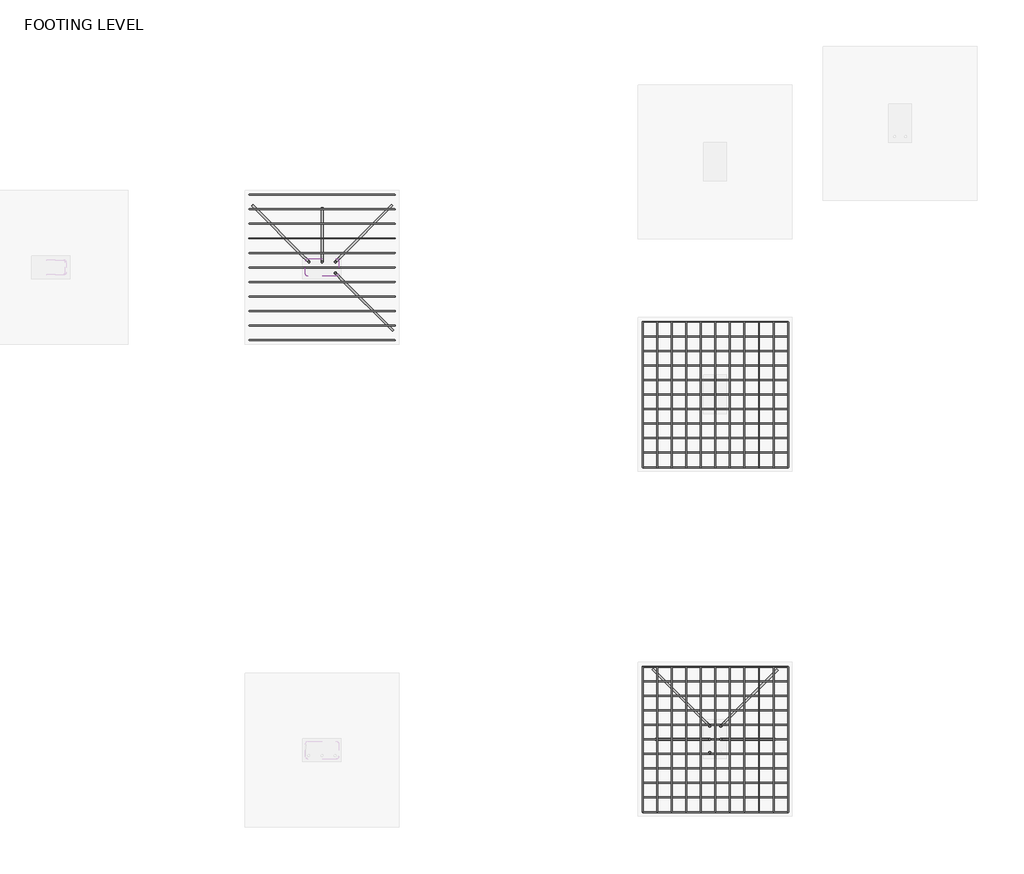
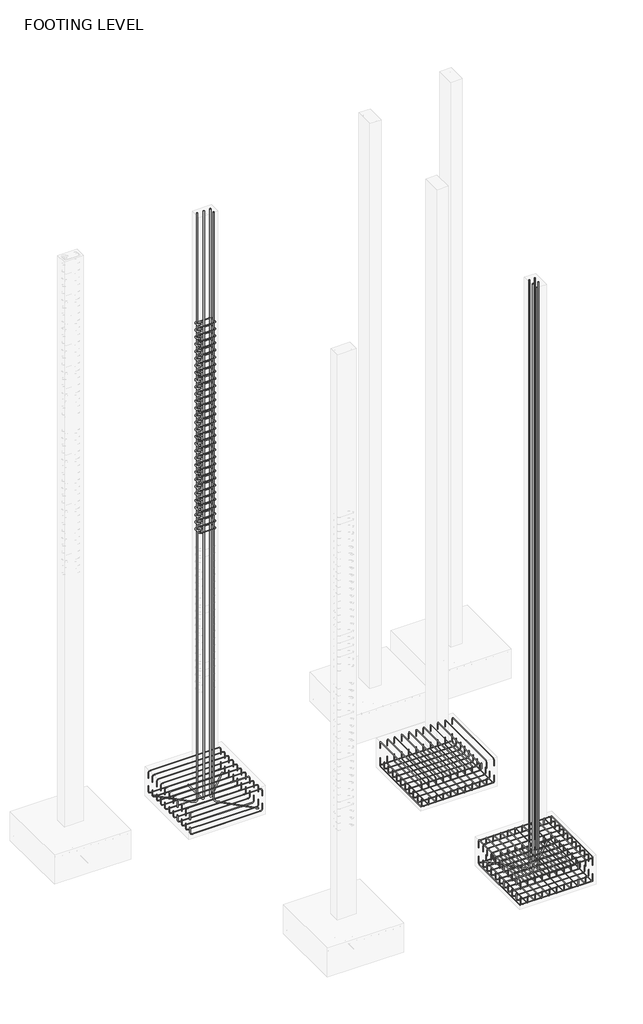
# One storey, part 5 of 10: 21 reinforcing bars.
"""IFC4 building model written with IfcOpenShell, lengths in millimetres."""

from ifc_helpers import new_model, si_unit, point, frame, origin, place, context, project, spatial, polyline, circle_curve, trimmed, segment, composite_curve, source, transform, mapped, element, save
from ifc_brep_helpers import swept_disk

model = new_model("IFC4")

# Units and contexts
model_context = context("Model", 3, world=origin())
ifc_project = project(units=[si_unit("LENGTHUNIT", "METRE", prefix="MILLI")], contexts=[model_context])

# Site, building, storey
site = spatial("IfcSite", under=ifc_project)
building = spatial("IfcBuilding", under=site)
storey = spatial("IfcBuildingStorey", under=building, Name="FOOTING LEVEL", Elevation=-1371.6)

# Reinforcing bars
placement = place(None, origin())
reinforcing_bar_shape = source(origin(), model_context, "Body", "SolidModel", [
    swept_disk(composite_curve([segment(polyline([(-7030.6793223, 2952.1203802, -1562.1), (-7030.6793223, 2952.1203802, -1447.8)]), True, "CONTINUOUS"), segment(trimmed(circle_curve(frame((-7030.6793223, 2985.4578802, -1447.8), z_axis=(-1.0, 0.0, 0.0), x_axis=(0.0, -33.33750000000009, 0.0)), 33.3375), [point((-7030.6793223, 2952.1203802, -1447.8))], [point((-7030.6793223, 2985.4578802, -1414.4625))], True, "CARTESIAN"), True, "CONTINUOUS"), segment(polyline([(-7030.6793223, 2985.4578802, -1414.4625), (-7030.6793223, 4357.0578802, -1414.4625)]), True, "CONTINUOUS"), segment(trimmed(circle_curve(frame((-7030.6793223, 4357.0578802, -1447.8), z_axis=(-1.0, 0.0, 0.0), x_axis=(0.0, 0.0, 33.337499999999864)), 33.3375), [point((-7030.6793223, 4357.0578802, -1414.4625))], [point((-7030.6793223, 4390.3953802, -1447.8))], True, "CARTESIAN"), True, "CONTINUOUS"), segment(polyline([(-7030.6793223, 4390.3953802, -1447.8), (-7030.6793223, 4390.3953802, -1562.1)]), True, "CONTINUOUS")], self_intersect=False), 4.7625),
])
element("IfcReinforcingBar", 1, at=placement, inside=storey, context=model_context, shape_type="MappedRepresentation", body=[
    mapped(reinforcing_bar_shape, transform((0.0, 0.0, 0.0), x_axis=(1.0, 0.0, 0.0), y_axis=(0.0, 1.0, 0.0), z_axis=(0.0, 0.0, 1.0))),
    mapped(reinforcing_bar_shape, transform((143.8275, 0.0, 0.0), x_axis=(1.0, 0.0, 0.0), y_axis=(0.0, 1.0, 0.0), z_axis=(0.0, 0.0, 1.0))),
    mapped(reinforcing_bar_shape, transform((287.655, 0.0, 0.0), x_axis=(1.0, 0.0, 0.0), y_axis=(0.0, 1.0, 0.0), z_axis=(0.0, 0.0, 1.0))),
    mapped(reinforcing_bar_shape, transform((431.4825, 0.0, 0.0), x_axis=(1.0, 0.0, 0.0), y_axis=(0.0, 1.0, 0.0), z_axis=(0.0, 0.0, 1.0))),
    mapped(reinforcing_bar_shape, transform((575.31, 0.0, 0.0), x_axis=(1.0, 0.0, 0.0), y_axis=(0.0, 1.0, 0.0), z_axis=(0.0, 0.0, 1.0))),
    mapped(reinforcing_bar_shape, transform((719.1375, 0.0, 0.0), x_axis=(1.0, 0.0, 0.0), y_axis=(0.0, 1.0, 0.0), z_axis=(0.0, 0.0, 1.0))),
    mapped(reinforcing_bar_shape, transform((862.965, 0.0, 0.0), x_axis=(1.0, 0.0, 0.0), y_axis=(0.0, 1.0, 0.0), z_axis=(0.0, 0.0, 1.0))),
    mapped(reinforcing_bar_shape, transform((1006.7925, 0.0, 0.0), x_axis=(1.0, 0.0, 0.0), y_axis=(0.0, 1.0, 0.0), z_axis=(0.0, 0.0, 1.0))),
    mapped(reinforcing_bar_shape, transform((1150.62, 0.0, 0.0), x_axis=(1.0, 0.0, 0.0), y_axis=(0.0, 1.0, 0.0), z_axis=(0.0, 0.0, 1.0))),
    mapped(reinforcing_bar_shape, transform((1294.4475, 0.0, 0.0), x_axis=(1.0, 0.0, 0.0), y_axis=(0.0, 1.0, 0.0), z_axis=(0.0, 0.0, 1.0))),
    mapped(reinforcing_bar_shape, transform((1438.275, 0.0, 0.0), x_axis=(1.0, 0.0, 0.0), y_axis=(0.0, 1.0, 0.0), z_axis=(0.0, 0.0, 1.0))),
])
reinforcing_bar_2_shape = source(origin(), model_context, "Body", "SolidModel", [
    swept_disk(composite_curve([segment(polyline([(-7030.6793223, 4390.3953802, -1790.7), (-7030.6793223, 4390.3953802, -1905.0)]), True, "CONTINUOUS"), segment(trimmed(circle_curve(frame((-7030.6793223, 4357.0578802, -1905.0), z_axis=(-1.0, 0.0, 0.0), x_axis=(0.0, 33.337499999999636, 0.0)), 33.3375), [point((-7030.6793223, 4390.3953802, -1905.0))], [point((-7030.6793223, 4357.0578802, -1938.3375))], True, "CARTESIAN"), True, "CONTINUOUS"), segment(polyline([(-7030.6793223, 4357.0578802, -1938.3375), (-7030.6793223, 2985.4578802, -1938.3375)]), True, "CONTINUOUS"), segment(trimmed(circle_curve(frame((-7030.6793223, 2985.4578802, -1905.0), z_axis=(-1.0, 0.0, 0.0), x_axis=(0.0, 0.0, -33.33750000000009)), 33.3375), [point((-7030.6793223, 2985.4578802, -1938.3375))], [point((-7030.6793223, 2952.1203802, -1905.0))], True, "CARTESIAN"), True, "CONTINUOUS"), segment(polyline([(-7030.6793223, 2952.1203802, -1905.0), (-7030.6793223, 2952.1203802, -1790.7)]), True, "CONTINUOUS")], self_intersect=False), 4.7625),
])
element("IfcReinforcingBar", 2, at=placement, inside=storey, context=model_context, shape_type="MappedRepresentation", body=[
    mapped(reinforcing_bar_2_shape, transform((0.0, 0.0, 0.0), x_axis=(1.0, 0.0, 0.0), y_axis=(0.0, 1.0, 0.0), z_axis=(0.0, 0.0, 1.0))),
    mapped(reinforcing_bar_2_shape, transform((143.8275, 0.0, 0.0), x_axis=(1.0, 0.0, 0.0), y_axis=(0.0, 1.0, 0.0), z_axis=(0.0, 0.0, 1.0))),
    mapped(reinforcing_bar_2_shape, transform((287.655, 0.0, 0.0), x_axis=(1.0, 0.0, 0.0), y_axis=(0.0, 1.0, 0.0), z_axis=(0.0, 0.0, 1.0))),
    mapped(reinforcing_bar_2_shape, transform((431.4825, 0.0, 0.0), x_axis=(1.0, 0.0, 0.0), y_axis=(0.0, 1.0, 0.0), z_axis=(0.0, 0.0, 1.0))),
    mapped(reinforcing_bar_2_shape, transform((575.31, 0.0, 0.0), x_axis=(1.0, 0.0, 0.0), y_axis=(0.0, 1.0, 0.0), z_axis=(0.0, 0.0, 1.0))),
    mapped(reinforcing_bar_2_shape, transform((719.1375, 0.0, 0.0), x_axis=(1.0, 0.0, 0.0), y_axis=(0.0, 1.0, 0.0), z_axis=(0.0, 0.0, 1.0))),
    mapped(reinforcing_bar_2_shape, transform((862.965, 0.0, 0.0), x_axis=(1.0, 0.0, 0.0), y_axis=(0.0, 1.0, 0.0), z_axis=(0.0, 0.0, 1.0))),
    mapped(reinforcing_bar_2_shape, transform((1006.7925, 0.0, 0.0), x_axis=(1.0, 0.0, 0.0), y_axis=(0.0, 1.0, 0.0), z_axis=(0.0, 0.0, 1.0))),
    mapped(reinforcing_bar_2_shape, transform((1150.62, 0.0, 0.0), x_axis=(1.0, 0.0, 0.0), y_axis=(0.0, 1.0, 0.0), z_axis=(0.0, 0.0, 1.0))),
    mapped(reinforcing_bar_2_shape, transform((1294.4475, 0.0, 0.0), x_axis=(1.0, 0.0, 0.0), y_axis=(0.0, 1.0, 0.0), z_axis=(0.0, 0.0, 1.0))),
    mapped(reinforcing_bar_2_shape, transform((1438.275, 0.0, 0.0), x_axis=(1.0, 0.0, 0.0), y_axis=(0.0, 1.0, 0.0), z_axis=(0.0, 0.0, 1.0))),
])
reinforcing_bar_3_shape = source(origin(), model_context, "Body", "SolidModel", [
    swept_disk(composite_curve([segment(polyline([(-5592.4043223, 4390.3953802, -1770.864029), (-5592.4043223, 4390.3953802, -1885.164029)]), True, "CONTINUOUS"), segment(trimmed(circle_curve(frame((-5625.7418223, 4390.3953802, -1885.164029), z_axis=(0.0, 1.0, 0.0), x_axis=(33.337500000000546, 0.0, 0.0)), 33.3375), [point((-5592.4043223, 4390.3953802, -1885.164029))], [point((-5625.7418223, 4390.3953802, -1918.501529))], True, "CARTESIAN"), True, "CONTINUOUS"), segment(polyline([(-5625.7418223, 4390.3953802, -1918.501529), (-6997.3418223, 4390.3953802, -1918.501529)]), True, "CONTINUOUS"), segment(trimmed(circle_curve(frame((-6997.3418223, 4390.3953802, -1885.164029), z_axis=(0.0, 1.0, 0.0), x_axis=(0.0, 0.0, -33.337499999999864)), 33.3375), [point((-6997.3418223, 4390.3953802, -1918.501529))], [point((-7030.6793223, 4390.3953802, -1885.164029))], True, "CARTESIAN"), True, "CONTINUOUS"), segment(polyline([(-7030.6793223, 4390.3953802, -1885.164029), (-7030.6793223, 4390.3953802, -1770.864029)]), True, "CONTINUOUS")], self_intersect=False), 4.7625),
])
element("IfcReinforcingBar", 3, at=placement, inside=storey, context=model_context, shape_type="MappedRepresentation", body=[
    mapped(reinforcing_bar_3_shape, transform((0.0, 0.0, 0.0), x_axis=(1.0, 0.0, 0.0), y_axis=(0.0, 1.0, 0.0), z_axis=(0.0, 0.0, 1.0))),
    mapped(reinforcing_bar_3_shape, transform((0.0, -143.8275, 0.0), x_axis=(1.0, 0.0, 0.0), y_axis=(0.0, 1.0, 0.0), z_axis=(0.0, 0.0, 1.0))),
    mapped(reinforcing_bar_3_shape, transform((0.0, -287.655, 0.0), x_axis=(1.0, 0.0, 0.0), y_axis=(0.0, 1.0, 0.0), z_axis=(0.0, 0.0, 1.0))),
    mapped(reinforcing_bar_3_shape, transform((0.0, -431.4825, 0.0), x_axis=(1.0, 0.0, 0.0), y_axis=(0.0, 1.0, 0.0), z_axis=(0.0, 0.0, 1.0))),
    mapped(reinforcing_bar_3_shape, transform((0.0, -575.31, 0.0), x_axis=(1.0, 0.0, 0.0), y_axis=(0.0, 1.0, 0.0), z_axis=(0.0, 0.0, 1.0))),
    mapped(reinforcing_bar_3_shape, transform((0.0, -719.1375, 0.0), x_axis=(1.0, 0.0, 0.0), y_axis=(0.0, 1.0, 0.0), z_axis=(0.0, 0.0, 1.0))),
    mapped(reinforcing_bar_3_shape, transform((0.0, -862.965, 0.0), x_axis=(1.0, 0.0, 0.0), y_axis=(0.0, 1.0, 0.0), z_axis=(0.0, 0.0, 1.0))),
    mapped(reinforcing_bar_3_shape, transform((0.0, -1006.7925, 0.0), x_axis=(1.0, 0.0, 0.0), y_axis=(0.0, 1.0, 0.0), z_axis=(0.0, 0.0, 1.0))),
    mapped(reinforcing_bar_3_shape, transform((0.0, -1150.62, 0.0), x_axis=(1.0, 0.0, 0.0), y_axis=(0.0, 1.0, 0.0), z_axis=(0.0, 0.0, 1.0))),
    mapped(reinforcing_bar_3_shape, transform((0.0, -1294.4475, 0.0), x_axis=(1.0, 0.0, 0.0), y_axis=(0.0, 1.0, 0.0), z_axis=(0.0, 0.0, 1.0))),
    mapped(reinforcing_bar_3_shape, transform((0.0, -1438.275, 0.0), x_axis=(1.0, 0.0, 0.0), y_axis=(0.0, 1.0, 0.0), z_axis=(0.0, 0.0, 1.0))),
])
reinforcing_bar_4_shape = source(origin(), model_context, "Body", "SolidModel", [
    swept_disk(composite_curve([segment(polyline([(-7030.6793223, -457.8296198, -1562.1), (-7030.6793223, -457.8296198, -1447.8)]), True, "CONTINUOUS"), segment(trimmed(circle_curve(frame((-7030.6793223, -424.4921198, -1447.8), z_axis=(-1.0, 0.0, 0.0), x_axis=(0.0, -33.33749999999998, 0.0)), 33.3375), [point((-7030.6793223, -457.8296198, -1447.8))], [point((-7030.6793223, -424.4921198, -1414.4625))], True, "CARTESIAN"), True, "CONTINUOUS"), segment(polyline([(-7030.6793223, -424.4921198, -1414.4625), (-7030.6793223, 947.1078802, -1414.4625)]), True, "CONTINUOUS"), segment(trimmed(circle_curve(frame((-7030.6793223, 947.1078802, -1447.8), z_axis=(-1.0, 0.0, 0.0), x_axis=(0.0, 0.0, 33.337499999999864)), 33.3375), [point((-7030.6793223, 947.1078802, -1414.4625))], [point((-7030.6793223, 980.4453802, -1447.8))], True, "CARTESIAN"), True, "CONTINUOUS"), segment(polyline([(-7030.6793223, 980.4453802, -1447.8), (-7030.6793223, 980.4453802, -1562.1)]), True, "CONTINUOUS")], self_intersect=False), 4.7625),
])
element("IfcReinforcingBar", 4, at=placement, inside=storey, context=model_context, shape_type="MappedRepresentation", body=[
    mapped(reinforcing_bar_4_shape, transform((0.0, 0.0, 0.0), x_axis=(1.0, 0.0, 0.0), y_axis=(0.0, 1.0, 0.0), z_axis=(0.0, 0.0, 1.0))),
    mapped(reinforcing_bar_4_shape, transform((143.8275, 0.0, 0.0), x_axis=(1.0, 0.0, 0.0), y_axis=(0.0, 1.0, 0.0), z_axis=(0.0, 0.0, 1.0))),
    mapped(reinforcing_bar_4_shape, transform((287.655, 0.0, 0.0), x_axis=(1.0, 0.0, 0.0), y_axis=(0.0, 1.0, 0.0), z_axis=(0.0, 0.0, 1.0))),
    mapped(reinforcing_bar_4_shape, transform((431.4825, 0.0, 0.0), x_axis=(1.0, 0.0, 0.0), y_axis=(0.0, 1.0, 0.0), z_axis=(0.0, 0.0, 1.0))),
    mapped(reinforcing_bar_4_shape, transform((575.31, 0.0, 0.0), x_axis=(1.0, 0.0, 0.0), y_axis=(0.0, 1.0, 0.0), z_axis=(0.0, 0.0, 1.0))),
    mapped(reinforcing_bar_4_shape, transform((719.1375, 0.0, 0.0), x_axis=(1.0, 0.0, 0.0), y_axis=(0.0, 1.0, 0.0), z_axis=(0.0, 0.0, 1.0))),
    mapped(reinforcing_bar_4_shape, transform((862.965, 0.0, 0.0), x_axis=(1.0, 0.0, 0.0), y_axis=(0.0, 1.0, 0.0), z_axis=(0.0, 0.0, 1.0))),
    mapped(reinforcing_bar_4_shape, transform((1006.7925, 0.0, 0.0), x_axis=(1.0, 0.0, 0.0), y_axis=(0.0, 1.0, 0.0), z_axis=(0.0, 0.0, 1.0))),
    mapped(reinforcing_bar_4_shape, transform((1150.62, 0.0, 0.0), x_axis=(1.0, 0.0, 0.0), y_axis=(0.0, 1.0, 0.0), z_axis=(0.0, 0.0, 1.0))),
    mapped(reinforcing_bar_4_shape, transform((1294.4475, 0.0, 0.0), x_axis=(1.0, 0.0, 0.0), y_axis=(0.0, 1.0, 0.0), z_axis=(0.0, 0.0, 1.0))),
    mapped(reinforcing_bar_4_shape, transform((1438.275, 0.0, 0.0), x_axis=(1.0, 0.0, 0.0), y_axis=(0.0, 1.0, 0.0), z_axis=(0.0, 0.0, 1.0))),
])
reinforcing_bar_5_shape = source(origin(), model_context, "Body", "SolidModel", [
    swept_disk(composite_curve([segment(polyline([(-7030.6793223, 980.4453802, -1790.7), (-7030.6793223, 980.4453802, -1905.0)]), True, "CONTINUOUS"), segment(trimmed(circle_curve(frame((-7030.6793223, 947.1078802, -1905.0), z_axis=(-1.0, 0.0, 0.0), x_axis=(0.0, 33.33750000000009, 0.0)), 33.3375), [point((-7030.6793223, 980.4453802, -1905.0))], [point((-7030.6793223, 947.1078802, -1938.3375))], True, "CARTESIAN"), True, "CONTINUOUS"), segment(polyline([(-7030.6793223, 947.1078802, -1938.3375), (-7030.6793223, -424.4921198, -1938.3375)]), True, "CONTINUOUS"), segment(trimmed(circle_curve(frame((-7030.6793223, -424.4921198, -1905.0), z_axis=(-1.0, 0.0, 0.0), x_axis=(0.0, 0.0, -33.33750000000009)), 33.3375), [point((-7030.6793223, -424.4921198, -1938.3375))], [point((-7030.6793223, -457.8296198, -1905.0))], True, "CARTESIAN"), True, "CONTINUOUS"), segment(polyline([(-7030.6793223, -457.8296198, -1905.0), (-7030.6793223, -457.8296198, -1790.7)]), True, "CONTINUOUS")], self_intersect=False), 4.7625),
])
element("IfcReinforcingBar", 5, at=placement, inside=storey, context=model_context, shape_type="MappedRepresentation", body=[
    mapped(reinforcing_bar_5_shape, transform((0.0, 0.0, 0.0), x_axis=(1.0, 0.0, 0.0), y_axis=(0.0, 1.0, 0.0), z_axis=(0.0, 0.0, 1.0))),
    mapped(reinforcing_bar_5_shape, transform((143.8275, 0.0, 0.0), x_axis=(1.0, 0.0, 0.0), y_axis=(0.0, 1.0, 0.0), z_axis=(0.0, 0.0, 1.0))),
    mapped(reinforcing_bar_5_shape, transform((287.655, 0.0, 0.0), x_axis=(1.0, 0.0, 0.0), y_axis=(0.0, 1.0, 0.0), z_axis=(0.0, 0.0, 1.0))),
    mapped(reinforcing_bar_5_shape, transform((431.4825, 0.0, 0.0), x_axis=(1.0, 0.0, 0.0), y_axis=(0.0, 1.0, 0.0), z_axis=(0.0, 0.0, 1.0))),
    mapped(reinforcing_bar_5_shape, transform((575.31, 0.0, 0.0), x_axis=(1.0, 0.0, 0.0), y_axis=(0.0, 1.0, 0.0), z_axis=(0.0, 0.0, 1.0))),
    mapped(reinforcing_bar_5_shape, transform((719.1375, 0.0, 0.0), x_axis=(1.0, 0.0, 0.0), y_axis=(0.0, 1.0, 0.0), z_axis=(0.0, 0.0, 1.0))),
    mapped(reinforcing_bar_5_shape, transform((862.965, 0.0, 0.0), x_axis=(1.0, 0.0, 0.0), y_axis=(0.0, 1.0, 0.0), z_axis=(0.0, 0.0, 1.0))),
    mapped(reinforcing_bar_5_shape, transform((1006.7925, 0.0, 0.0), x_axis=(1.0, 0.0, 0.0), y_axis=(0.0, 1.0, 0.0), z_axis=(0.0, 0.0, 1.0))),
    mapped(reinforcing_bar_5_shape, transform((1150.62, 0.0, 0.0), x_axis=(1.0, 0.0, 0.0), y_axis=(0.0, 1.0, 0.0), z_axis=(0.0, 0.0, 1.0))),
    mapped(reinforcing_bar_5_shape, transform((1294.4475, 0.0, 0.0), x_axis=(1.0, 0.0, 0.0), y_axis=(0.0, 1.0, 0.0), z_axis=(0.0, 0.0, 1.0))),
    mapped(reinforcing_bar_5_shape, transform((1438.275, 0.0, 0.0), x_axis=(1.0, 0.0, 0.0), y_axis=(0.0, 1.0, 0.0), z_axis=(0.0, 0.0, 1.0))),
])
reinforcing_bar_6_shape = source(origin(), model_context, "Body", "SolidModel", [
    swept_disk(composite_curve([segment(polyline([(-5592.4043223, 980.4453802, -1770.864029), (-5592.4043223, 980.4453802, -1885.164029)]), True, "CONTINUOUS"), segment(trimmed(circle_curve(frame((-5625.7418223, 980.4453802, -1885.164029), z_axis=(0.0, 1.0, 0.0), x_axis=(33.337500000000546, 0.0, 0.0)), 33.3375), [point((-5592.4043223, 980.4453802, -1885.164029))], [point((-5625.7418223, 980.4453802, -1918.501529))], True, "CARTESIAN"), True, "CONTINUOUS"), segment(polyline([(-5625.7418223, 980.4453802, -1918.501529), (-6997.3418223, 980.4453802, -1918.501529)]), True, "CONTINUOUS"), segment(trimmed(circle_curve(frame((-6997.3418223, 980.4453802, -1885.164029), z_axis=(0.0, 1.0, 0.0), x_axis=(0.0, 0.0, -33.337499999999864)), 33.3375), [point((-6997.3418223, 980.4453802, -1918.501529))], [point((-7030.6793223, 980.4453802, -1885.164029))], True, "CARTESIAN"), True, "CONTINUOUS"), segment(polyline([(-7030.6793223, 980.4453802, -1885.164029), (-7030.6793223, 980.4453802, -1770.864029)]), True, "CONTINUOUS")], self_intersect=False), 4.7625),
])
element("IfcReinforcingBar", 6, at=placement, inside=storey, context=model_context, shape_type="MappedRepresentation", body=[
    mapped(reinforcing_bar_6_shape, transform((0.0, 0.0, 0.0), x_axis=(1.0, 0.0, 0.0), y_axis=(0.0, 1.0, 0.0), z_axis=(0.0, 0.0, 1.0))),
    mapped(reinforcing_bar_6_shape, transform((0.0, -143.8275, 0.0), x_axis=(1.0, 0.0, 0.0), y_axis=(0.0, 1.0, 0.0), z_axis=(0.0, 0.0, 1.0))),
    mapped(reinforcing_bar_6_shape, transform((0.0, -287.655, 0.0), x_axis=(1.0, 0.0, 0.0), y_axis=(0.0, 1.0, 0.0), z_axis=(0.0, 0.0, 1.0))),
    mapped(reinforcing_bar_6_shape, transform((0.0, -431.4825, 0.0), x_axis=(1.0, 0.0, 0.0), y_axis=(0.0, 1.0, 0.0), z_axis=(0.0, 0.0, 1.0))),
    mapped(reinforcing_bar_6_shape, transform((0.0, -575.31, 0.0), x_axis=(1.0, 0.0, 0.0), y_axis=(0.0, 1.0, 0.0), z_axis=(0.0, 0.0, 1.0))),
    mapped(reinforcing_bar_6_shape, transform((0.0, -719.1375, 0.0), x_axis=(1.0, 0.0, 0.0), y_axis=(0.0, 1.0, 0.0), z_axis=(0.0, 0.0, 1.0))),
    mapped(reinforcing_bar_6_shape, transform((0.0, -862.965, 0.0), x_axis=(1.0, 0.0, 0.0), y_axis=(0.0, 1.0, 0.0), z_axis=(0.0, 0.0, 1.0))),
    mapped(reinforcing_bar_6_shape, transform((0.0, -1006.7925, 0.0), x_axis=(1.0, 0.0, 0.0), y_axis=(0.0, 1.0, 0.0), z_axis=(0.0, 0.0, 1.0))),
    mapped(reinforcing_bar_6_shape, transform((0.0, -1150.62, 0.0), x_axis=(1.0, 0.0, 0.0), y_axis=(0.0, 1.0, 0.0), z_axis=(0.0, 0.0, 1.0))),
    mapped(reinforcing_bar_6_shape, transform((0.0, -1294.4475, 0.0), x_axis=(1.0, 0.0, 0.0), y_axis=(0.0, 1.0, 0.0), z_axis=(0.0, 0.0, 1.0))),
    mapped(reinforcing_bar_6_shape, transform((0.0, -1438.275, 0.0), x_axis=(1.0, 0.0, 0.0), y_axis=(0.0, 1.0, 0.0), z_axis=(0.0, 0.0, 1.0))),
])
reinforcing_bar_7_shape = source(origin(), model_context, "Body", "SolidModel", [
    swept_disk(composite_curve([segment(polyline([(-5592.4043223, -457.8296198, -1586.5406765), (-5592.4043223, -457.8296198, -1472.2406765)]), True, "CONTINUOUS"), segment(trimmed(circle_curve(frame((-5625.7418223, -457.8296198, -1472.2406765), z_axis=(0.0, -1.0, 0.0), x_axis=(33.337500000000546, 0.0, 0.0)), 33.3375), [point((-5592.4043223, -457.8296198, -1472.2406765))], [point((-5625.7418223, -457.8296198, -1438.9031765))], True, "CARTESIAN"), True, "CONTINUOUS"), segment(polyline([(-5625.7418223, -457.8296198, -1438.9031765), (-6997.3418223, -457.8296198, -1438.9031765)]), True, "CONTINUOUS"), segment(trimmed(circle_curve(frame((-6997.3418223, -457.8296198, -1472.2406765), z_axis=(0.0, -1.0, 0.0), x_axis=(0.0, 0.0, 33.33750000000009)), 33.3375), [point((-6997.3418223, -457.8296198, -1438.9031765))], [point((-7030.6793223, -457.8296198, -1472.2406765))], True, "CARTESIAN"), True, "CONTINUOUS"), segment(polyline([(-7030.6793223, -457.8296198, -1472.2406765), (-7030.6793223, -457.8296198, -1586.5406765)]), True, "CONTINUOUS")], self_intersect=False), 4.7625),
])
element("IfcReinforcingBar", 7, at=placement, inside=storey, context=model_context, shape_type="MappedRepresentation", body=[
    mapped(reinforcing_bar_7_shape, transform((0.0, 0.0, 0.0), x_axis=(1.0, 0.0, 0.0), y_axis=(0.0, 1.0, 0.0), z_axis=(0.0, 0.0, 1.0))),
    mapped(reinforcing_bar_7_shape, transform((0.0, 143.8275, 0.0), x_axis=(1.0, 0.0, 0.0), y_axis=(0.0, 1.0, 0.0), z_axis=(0.0, 0.0, 1.0))),
    mapped(reinforcing_bar_7_shape, transform((0.0, 287.655, 0.0), x_axis=(1.0, 0.0, 0.0), y_axis=(0.0, 1.0, 0.0), z_axis=(0.0, 0.0, 1.0))),
    mapped(reinforcing_bar_7_shape, transform((0.0, 431.4825, 0.0), x_axis=(1.0, 0.0, 0.0), y_axis=(0.0, 1.0, 0.0), z_axis=(0.0, 0.0, 1.0))),
    mapped(reinforcing_bar_7_shape, transform((0.0, 575.31, 0.0), x_axis=(1.0, 0.0, 0.0), y_axis=(0.0, 1.0, 0.0), z_axis=(0.0, 0.0, 1.0))),
    mapped(reinforcing_bar_7_shape, transform((0.0, 719.1375, 0.0), x_axis=(1.0, 0.0, 0.0), y_axis=(0.0, 1.0, 0.0), z_axis=(0.0, 0.0, 1.0))),
    mapped(reinforcing_bar_7_shape, transform((0.0, 862.965, 0.0), x_axis=(1.0, 0.0, 0.0), y_axis=(0.0, 1.0, 0.0), z_axis=(0.0, 0.0, 1.0))),
    mapped(reinforcing_bar_7_shape, transform((0.0, 1006.7925, 0.0), x_axis=(1.0, 0.0, 0.0), y_axis=(0.0, 1.0, 0.0), z_axis=(0.0, 0.0, 1.0))),
    mapped(reinforcing_bar_7_shape, transform((0.0, 1150.62, 0.0), x_axis=(1.0, 0.0, 0.0), y_axis=(0.0, 1.0, 0.0), z_axis=(0.0, 0.0, 1.0))),
    mapped(reinforcing_bar_7_shape, transform((0.0, 1294.4475, 0.0), x_axis=(1.0, 0.0, 0.0), y_axis=(0.0, 1.0, 0.0), z_axis=(0.0, 0.0, 1.0))),
    mapped(reinforcing_bar_7_shape, transform((0.0, 1438.275, 0.0), x_axis=(1.0, 0.0, 0.0), y_axis=(0.0, 1.0, 0.0), z_axis=(0.0, 0.0, 1.0))),
])
element("IfcReinforcingBar", 8, at=placement, inside=storey, context=model_context, shape_type="SolidModel", body=[
    swept_disk(composite_curve([segment(polyline([(-9505.5058743, 5544.1610861, -1910.4342608), (-10020.0352856, 5029.6316749, -1910.4342608)]), True, "CONTINUOUS"), segment(trimmed(circle_curve(frame((-10020.0352856, 5029.6316749, -1843.7592608), z_axis=(-0.7071067811865184, 0.7071067811865768, 0.0), x_axis=(0.0, 0.0, -66.67499999999995)), 66.675), [point((-10020.0352856, 5029.6316749, -1910.4342608))], [point((-10067.1816302, 4982.4853303, -1843.7592608))], True, "CARTESIAN"), True, "CONTINUOUS"), segment(polyline([(-10067.1816302, 4982.4853303, -1843.7592608), (-10067.1816302, 4982.4853303, 10490.2)]), True, "CONTINUOUS")], self_intersect=False), 9.525),
])
element("IfcReinforcingBar", 9, at=placement, inside=storey, context=model_context, shape_type="SolidModel", body=[
    swept_disk(composite_curve([segment(polyline([(-9497.4874965, 4304.0708123, -1910.4342608), (-10020.0352856, 4826.6186014, -1910.4342608)]), True, "CONTINUOUS"), segment(trimmed(circle_curve(frame((-10020.0352856, 4826.6186014, -1843.7592608), z_axis=(0.707106781186527, 0.707106781186568, 0.0), x_axis=(0.0, 0.0, -66.67499999999995)), 66.675), [point((-10020.0352856, 4826.6186014, -1910.4342608))], [point((-10067.1816302, 4873.7649461, -1843.7592608))], True, "CARTESIAN"), True, "CONTINUOUS"), segment(polyline([(-10067.1816302, 4873.7649461, -1843.7592608), (-10067.1816302, 4873.7649461, 10490.2)]), True, "CONTINUOUS")], self_intersect=False), 9.525),
])
element("IfcReinforcingBar", 10, at=placement, inside=storey, context=model_context, shape_type="SolidModel", body=[
    swept_disk(composite_curve([segment(polyline([(-10887.0211349, 5541.2044507, -1910.4342608), (-10375.4483591, 5029.6316749, -1910.4342608)]), True, "CONTINUOUS"), segment(trimmed(circle_curve(frame((-10375.4483591, 5029.6316749, -1843.7592608), z_axis=(-0.7071067811865224, -0.7071067811865728, 0.0), x_axis=(0.0, 0.0, -66.67499999999995)), 66.675), [point((-10375.4483591, 5029.6316749, -1910.4342608))], [point((-10328.3020144, 4982.4853303, -1843.7592608))], True, "CARTESIAN"), True, "CONTINUOUS"), segment(polyline([(-10328.3020144, 4982.4853303, -1843.7592608), (-10328.3020144, 4982.4853303, 10490.2)]), True, "CONTINUOUS")], self_intersect=False), 9.525),
])
element("IfcReinforcingBar", 11, at=placement, inside=storey, context=model_context, shape_type="SolidModel", body=[
    swept_disk(composite_curve([segment(polyline([(-10197.7418223, 5520.7152067, -1910.4342608), (-10197.7418223, 5049.1603303, -1910.4342608)]), True, "CONTINUOUS"), segment(trimmed(circle_curve(frame((-10197.7418223, 5049.1603303, -1843.7592608), z_axis=(-1.0, 0.0, 0.0), x_axis=(0.0, 0.0, -66.67499999999995)), 66.675), [point((-10197.7418223, 5049.1603303, -1910.4342608))], [point((-10197.7418223, 4982.4853303, -1843.7592608))], True, "CARTESIAN"), True, "CONTINUOUS"), segment(polyline([(-10197.7418223, 4982.4853303, -1843.7592608), (-10197.7418223, 4982.4853303, 10490.2)]), True, "CONTINUOUS")], self_intersect=False), 9.525),
])
element("IfcReinforcingBar", 12, at=placement, inside=storey, context=model_context, shape_type="SolidModel", body=[
    swept_disk(composite_curve([segment(polyline([(-6365.9020144, 130.7476881, -1333.5), (-6365.9020144, 130.7476881, 10477.5)]), True, "CONTINUOUS")], self_intersect=False), 9.525),
])
element("IfcReinforcingBar", 13, at=placement, inside=storey, context=model_context, shape_type="SolidModel", body=[
    swept_disk(composite_curve([segment(polyline([(-6257.1816302, 391.8680723, -1333.5), (-6257.1816302, 391.8680723, 10477.5)]), True, "CONTINUOUS")], self_intersect=False), 9.525),
])
element("IfcReinforcingBar", 14, at=placement, inside=storey, context=model_context, shape_type="SolidModel", body=[
    swept_disk(composite_curve([segment(polyline([(-6365.9020144, 391.8680723, -1333.5), (-6365.9020144, 391.8680723, 10477.5)]), True, "CONTINUOUS")], self_intersect=False), 9.525),
])
element("IfcReinforcingBar", 15, at=placement, inside=storey, context=model_context, shape_type="SolidModel", body=[
    swept_disk(composite_curve([segment(polyline([(-5698.4625098, 950.5871927, -1910.4342608), (-6210.0352856, 439.0144169, -1910.4342608)]), True, "CONTINUOUS"), segment(trimmed(circle_curve(frame((-6210.0352856, 439.0144169, -1843.7592608), z_axis=(-0.7071067811865738, 0.7071067811865214, 0.0), x_axis=(0.0, 0.0, -66.67499999999995)), 66.675), [point((-6210.0352856, 439.0144169, -1910.4342608))], [point((-6257.1816302, 391.8680723, -1843.7592608))], True, "CARTESIAN"), True, "CONTINUOUS"), segment(polyline([(-6257.1816302, 391.8680723, -1843.7592608), (-6257.1816302, 391.8680723, 10477.5)]), True, "CONTINUOUS")], self_intersect=False), 9.525),
])
element("IfcReinforcingBar", 16, at=placement, inside=storey, context=model_context, shape_type="SolidModel", body=[
    swept_disk(composite_curve([segment(polyline([(-6930.0808347, 956.0468926, -1910.4342608), (-6413.048359, 439.0144169, -1910.4342608)]), True, "CONTINUOUS"), segment(trimmed(circle_curve(frame((-6413.048359, 439.0144169, -1843.7592608), z_axis=(-0.7071067811865711, -0.7071067811865239, 0.0), x_axis=(0.0, 0.0, -66.67499999999995)), 66.675), [point((-6413.048359, 439.0144169, -1910.4342608))], [point((-6365.9020144, 391.8680723, -1843.7592608))], True, "CARTESIAN"), True, "CONTINUOUS"), segment(polyline([(-6365.9020144, 391.8680723, -1843.7592608), (-6365.9020144, 391.8680723, 10477.5)]), True, "CONTINUOUS")], self_intersect=False), 9.525),
])
element("IfcReinforcingBar", 17, at=placement, inside=storey, context=model_context, shape_type="SolidModel", body=[
    swept_disk(composite_curve([segment(polyline([(-5718.9517538, 261.3078802, -1910.4342608), (-6190.5066302, 261.3078802, -1910.4342608)]), True, "CONTINUOUS"), segment(trimmed(circle_curve(frame((-6190.5066302, 261.3078802, -1843.7592608), z_axis=(0.0, 1.0, 0.0), x_axis=(0.0, 0.0, -66.67499999999995)), 66.675), [point((-6190.5066302, 261.3078802, -1910.4342608))], [point((-6257.1816302, 261.3078802, -1843.7592608))], True, "CARTESIAN"), True, "CONTINUOUS"), segment(polyline([(-6257.1816302, 261.3078802, -1843.7592608), (-6257.1816302, 261.3078802, 10477.5)]), True, "CONTINUOUS")], self_intersect=False), 9.525),
])
element("IfcReinforcingBar", 18, at=placement, inside=storey, context=model_context, shape_type="SolidModel", body=[
    swept_disk(composite_curve([segment(polyline([(-6904.1318909, 261.3078802, -1910.4342608), (-6432.5770144, 261.3078802, -1910.4342608)]), True, "CONTINUOUS"), segment(trimmed(circle_curve(frame((-6432.5770144, 261.3078802, -1843.7592608), z_axis=(0.0, -1.0, 0.0), x_axis=(0.0, 0.0, -66.67499999999995)), 66.675), [point((-6432.5770144, 261.3078802, -1910.4342608))], [point((-6365.9020144, 261.3078802, -1843.7592608))], True, "CARTESIAN"), True, "CONTINUOUS"), segment(polyline([(-6365.9020144, 261.3078802, -1843.7592608), (-6365.9020144, 261.3078802, 10477.5)]), True, "CONTINUOUS")], self_intersect=False), 9.525),
])
reinforcing_bar_8_shape = source(origin(), model_context, "Body", "SolidModel", [
    swept_disk(composite_curve([segment(polyline([(-10260.564645, 4948.4239213, 3844.2488128), (-10317.4288421, 5005.2881184, 3844.2488128)]), True, "CONTINUOUS"), segment(trimmed(circle_curve(frame((-10334.2668223, 4988.4501382, 3844.2488128), z_axis=(0.0, 0.0, 1.0), x_axis=(16.837980199999947, 16.837980199999947, 0.0)), 23.8125), [point((-10317.4288421, 5005.2881184, 3844.2488128))], [point((-10358.0793223, 4988.4501382, 3844.2488128))], True, "CARTESIAN"), True, "CONTINUOUS"), segment(polyline([(-10358.0793223, 4988.4501382, 3844.2488128), (-10358.0793223, 4867.8001382, 3844.2488128)]), True, "CONTINUOUS"), segment(trimmed(circle_curve(frame((-10334.2668223, 4867.8001382, 3844.2488128), z_axis=(0.0, 0.0, 1.0), x_axis=(-23.8125, 0.0, 0.0)), 23.8125), [point((-10358.0793223, 4867.8001382, 3844.2488128))], [point((-10334.2668223, 4843.9876382, 3844.2488128))], True, "CARTESIAN"), True, "CONTINUOUS"), segment(polyline([(-10334.2668223, 4843.9876382, 3844.2488128), (-10061.2168223, 4843.9876382, 3844.2488128)]), True, "CONTINUOUS"), segment(trimmed(circle_curve(frame((-10061.2168223, 4867.7620821, 3842.9030896), z_axis=(0.0, 0.056513312022656075, 0.9984018457335854), x_axis=(0.0, -23.774443899999824, 1.3457232000000658)), 23.8125), [point((-10061.2168223, 4843.9876382, 3844.2488128))], [point((-10037.4043223, 4867.7620821, 3842.9030896))], True, "CARTESIAN"), True, "CONTINUOUS"), segment(polyline([(-10037.4043223, 4867.7620821, 3842.9030896), (-10037.4043223, 4988.4881942, 3836.0695361)]), True, "CONTINUOUS"), segment(trimmed(circle_curve(frame((-10061.2168223, 4988.4881942, 3836.0695361), z_axis=(0.0, 0.056513312022656075, 0.9984018457335854), x_axis=(23.8125, 0.0, 0.0)), 23.8125), [point((-10037.4043223, 4988.4881942, 3836.0695361))], [point((-10061.2168223, 5012.2626382, 3834.7238128))], True, "CARTESIAN"), True, "CONTINUOUS"), segment(polyline([(-10061.2168223, 5012.2626382, 3834.7238128), (-10334.2668223, 5012.2626382, 3834.7238128)]), True, "CONTINUOUS"), segment(trimmed(circle_curve(frame((-10334.2668223, 4988.4501382, 3834.7238128), z_axis=(0.0, 0.0, 1.0), x_axis=(0.0, 23.8125, 0.0)), 23.8125), [point((-10334.2668223, 5012.2626382, 3834.7238128))], [point((-10351.1048026, 4971.6121579, 3834.7238128))], True, "CARTESIAN"), True, "CONTINUOUS"), segment(polyline([(-10351.1048026, 4971.6121579, 3834.7238128), (-10294.2406055, 4914.7479609, 3834.7238128)]), True, "CONTINUOUS")], self_intersect=False), 4.7625),
])
element("IfcReinforcingBar", 19, at=placement, inside=storey, context=model_context, shape_type="MappedRepresentation", body=[
    mapped(reinforcing_bar_8_shape, transform((0.0, 0.0, 0.0), x_axis=(1.0, 0.0, 0.0), y_axis=(0.0, 1.0, 0.0), z_axis=(0.0, 0.0, 1.0))),
    mapped(reinforcing_bar_8_shape, transform((0.0, 0.0, 149.5868115), x_axis=(1.0, 0.0, 0.0), y_axis=(0.0, 1.0, 0.0), z_axis=(0.0, 0.0, 1.0))),
    mapped(reinforcing_bar_8_shape, transform((0.0, 0.0, 299.173623), x_axis=(1.0, 0.0, 0.0), y_axis=(0.0, 1.0, 0.0), z_axis=(0.0, 0.0, 1.0))),
    mapped(reinforcing_bar_8_shape, transform((0.0, 0.0, 448.7604345), x_axis=(1.0, 0.0, 0.0), y_axis=(0.0, 1.0, 0.0), z_axis=(0.0, 0.0, 1.0))),
    mapped(reinforcing_bar_8_shape, transform((0.0, 0.0, 598.347246), x_axis=(1.0, 0.0, 0.0), y_axis=(0.0, 1.0, 0.0), z_axis=(0.0, 0.0, 1.0))),
    mapped(reinforcing_bar_8_shape, transform((0.0, 0.0, 747.9340575), x_axis=(1.0, 0.0, 0.0), y_axis=(0.0, 1.0, 0.0), z_axis=(0.0, 0.0, 1.0))),
    mapped(reinforcing_bar_8_shape, transform((0.0, 0.0, 897.520869), x_axis=(1.0, 0.0, 0.0), y_axis=(0.0, 1.0, 0.0), z_axis=(0.0, 0.0, 1.0))),
    mapped(reinforcing_bar_8_shape, transform((0.0, 0.0, 1047.1076805), x_axis=(1.0, 0.0, 0.0), y_axis=(0.0, 1.0, 0.0), z_axis=(0.0, 0.0, 1.0))),
    mapped(reinforcing_bar_8_shape, transform((0.0, 0.0, 1196.694492), x_axis=(1.0, 0.0, 0.0), y_axis=(0.0, 1.0, 0.0), z_axis=(0.0, 0.0, 1.0))),
    mapped(reinforcing_bar_8_shape, transform((0.0, 0.0, 1346.2813035), x_axis=(1.0, 0.0, 0.0), y_axis=(0.0, 1.0, 0.0), z_axis=(0.0, 0.0, 1.0))),
    mapped(reinforcing_bar_8_shape, transform((0.0, 0.0, 1495.868115), x_axis=(1.0, 0.0, 0.0), y_axis=(0.0, 1.0, 0.0), z_axis=(0.0, 0.0, 1.0))),
    mapped(reinforcing_bar_8_shape, transform((0.0, 0.0, 1645.4549265), x_axis=(1.0, 0.0, 0.0), y_axis=(0.0, 1.0, 0.0), z_axis=(0.0, 0.0, 1.0))),
    mapped(reinforcing_bar_8_shape, transform((0.0, 0.0, 1795.041738), x_axis=(1.0, 0.0, 0.0), y_axis=(0.0, 1.0, 0.0), z_axis=(0.0, 0.0, 1.0))),
    mapped(reinforcing_bar_8_shape, transform((0.0, 0.0, 1944.6285495), x_axis=(1.0, 0.0, 0.0), y_axis=(0.0, 1.0, 0.0), z_axis=(0.0, 0.0, 1.0))),
    mapped(reinforcing_bar_8_shape, transform((0.0, 0.0, 2094.215361), x_axis=(1.0, 0.0, 0.0), y_axis=(0.0, 1.0, 0.0), z_axis=(0.0, 0.0, 1.0))),
    mapped(reinforcing_bar_8_shape, transform((0.0, 0.0, 2243.8021725), x_axis=(1.0, 0.0, 0.0), y_axis=(0.0, 1.0, 0.0), z_axis=(0.0, 0.0, 1.0))),
    mapped(reinforcing_bar_8_shape, transform((0.0, 0.0, 2393.388984), x_axis=(1.0, 0.0, 0.0), y_axis=(0.0, 1.0, 0.0), z_axis=(0.0, 0.0, 1.0))),
    mapped(reinforcing_bar_8_shape, transform((0.0, 0.0, 2542.9757955), x_axis=(1.0, 0.0, 0.0), y_axis=(0.0, 1.0, 0.0), z_axis=(0.0, 0.0, 1.0))),
    mapped(reinforcing_bar_8_shape, transform((0.0, 0.0, 2692.562607), x_axis=(1.0, 0.0, 0.0), y_axis=(0.0, 1.0, 0.0), z_axis=(0.0, 0.0, 1.0))),
    mapped(reinforcing_bar_8_shape, transform((0.0, 0.0, 2842.1494185), x_axis=(1.0, 0.0, 0.0), y_axis=(0.0, 1.0, 0.0), z_axis=(0.0, 0.0, 1.0))),
    mapped(reinforcing_bar_8_shape, transform((0.0, 0.0, 2991.73623), x_axis=(1.0, 0.0, 0.0), y_axis=(0.0, 1.0, 0.0), z_axis=(0.0, 0.0, 1.0))),
    mapped(reinforcing_bar_8_shape, transform((0.0, 0.0, 3141.3230415), x_axis=(1.0, 0.0, 0.0), y_axis=(0.0, 1.0, 0.0), z_axis=(0.0, 0.0, 1.0))),
    mapped(reinforcing_bar_8_shape, transform((0.0, 0.0, 3290.909853), x_axis=(1.0, 0.0, 0.0), y_axis=(0.0, 1.0, 0.0), z_axis=(0.0, 0.0, 1.0))),
    mapped(reinforcing_bar_8_shape, transform((0.0, 0.0, 3440.4966645), x_axis=(1.0, 0.0, 0.0), y_axis=(0.0, 1.0, 0.0), z_axis=(0.0, 0.0, 1.0))),
    mapped(reinforcing_bar_8_shape, transform((0.0, 0.0, 3590.083476), x_axis=(1.0, 0.0, 0.0), y_axis=(0.0, 1.0, 0.0), z_axis=(0.0, 0.0, 1.0))),
    mapped(reinforcing_bar_8_shape, transform((0.0, 0.0, 3739.6702875), x_axis=(1.0, 0.0, 0.0), y_axis=(0.0, 1.0, 0.0), z_axis=(0.0, 0.0, 1.0))),
    mapped(reinforcing_bar_8_shape, transform((0.0, 0.0, 3889.257099), x_axis=(1.0, 0.0, 0.0), y_axis=(0.0, 1.0, 0.0), z_axis=(0.0, 0.0, 1.0))),
    mapped(reinforcing_bar_8_shape, transform((0.0, 0.0, 4038.8439105), x_axis=(1.0, 0.0, 0.0), y_axis=(0.0, 1.0, 0.0), z_axis=(0.0, 0.0, 1.0))),
    mapped(reinforcing_bar_8_shape, transform((0.0, 0.0, 4188.430722), x_axis=(1.0, 0.0, 0.0), y_axis=(0.0, 1.0, 0.0), z_axis=(0.0, 0.0, 1.0))),
    mapped(reinforcing_bar_8_shape, transform((0.0, 0.0, 4338.0175335), x_axis=(1.0, 0.0, 0.0), y_axis=(0.0, 1.0, 0.0), z_axis=(0.0, 0.0, 1.0))),
])
reinforcing_bar_9_shape = source(origin(), model_context, "Body", "SolidModel", [
    swept_disk(composite_curve([segment(polyline([(-10916.8793223, 4208.9876382, -1760.6672682), (-10916.8793223, 4208.9876382, -1874.9672682)]), True, "CONTINUOUS"), segment(trimmed(circle_curve(frame((-10883.5418223, 4208.9876382, -1874.9672682), z_axis=(0.0, -1.0, 0.0), x_axis=(-33.337499999999636, 0.0, 0.0)), 33.3375), [point((-10916.8793223, 4208.9876382, -1874.9672682))], [point((-10883.5418223, 4208.9876382, -1908.3047682))], True, "CARTESIAN"), True, "CONTINUOUS"), segment(polyline([(-10883.5418223, 4208.9876382, -1908.3047682), (-9511.9418223, 4208.9876382, -1908.3047682)]), True, "CONTINUOUS"), segment(trimmed(circle_curve(frame((-9511.9418223, 4208.9876382, -1874.9672682), z_axis=(0.0, -1.0, 0.0), x_axis=(0.0, 0.0, -33.337499999999864)), 33.3375), [point((-9511.9418223, 4208.9876382, -1908.3047682))], [point((-9478.6043223, 4208.9876382, -1874.9672682))], True, "CARTESIAN"), True, "CONTINUOUS"), segment(polyline([(-9478.6043223, 4208.9876382, -1874.9672682), (-9478.6043223, 4208.9876382, -1760.6672682)]), True, "CONTINUOUS")], self_intersect=False), 4.7625),
])
element("IfcReinforcingBar", 20, at=placement, inside=storey, context=model_context, shape_type="MappedRepresentation", body=[
    mapped(reinforcing_bar_9_shape, transform((0.0, 0.0, 0.0), x_axis=(1.0, 0.0, 0.0), y_axis=(0.0, 1.0, 0.0), z_axis=(0.0, 0.0, 1.0))),
    mapped(reinforcing_bar_9_shape, transform((0.0, 143.8275, 0.0), x_axis=(1.0, 0.0, 0.0), y_axis=(0.0, 1.0, 0.0), z_axis=(0.0, 0.0, 1.0))),
    mapped(reinforcing_bar_9_shape, transform((0.0, 287.655, 0.0), x_axis=(1.0, 0.0, 0.0), y_axis=(0.0, 1.0, 0.0), z_axis=(0.0, 0.0, 1.0))),
    mapped(reinforcing_bar_9_shape, transform((0.0, 431.4825, 0.0), x_axis=(1.0, 0.0, 0.0), y_axis=(0.0, 1.0, 0.0), z_axis=(0.0, 0.0, 1.0))),
    mapped(reinforcing_bar_9_shape, transform((0.0, 575.31, 0.0), x_axis=(1.0, 0.0, 0.0), y_axis=(0.0, 1.0, 0.0), z_axis=(0.0, 0.0, 1.0))),
    mapped(reinforcing_bar_9_shape, transform((0.0, 719.1375, 0.0), x_axis=(1.0, 0.0, 0.0), y_axis=(0.0, 1.0, 0.0), z_axis=(0.0, 0.0, 1.0))),
    mapped(reinforcing_bar_9_shape, transform((0.0, 862.965, 0.0), x_axis=(1.0, 0.0, 0.0), y_axis=(0.0, 1.0, 0.0), z_axis=(0.0, 0.0, 1.0))),
    mapped(reinforcing_bar_9_shape, transform((0.0, 1006.7925, 0.0), x_axis=(1.0, 0.0, 0.0), y_axis=(0.0, 1.0, 0.0), z_axis=(0.0, 0.0, 1.0))),
    mapped(reinforcing_bar_9_shape, transform((0.0, 1150.62, 0.0), x_axis=(1.0, 0.0, 0.0), y_axis=(0.0, 1.0, 0.0), z_axis=(0.0, 0.0, 1.0))),
    mapped(reinforcing_bar_9_shape, transform((0.0, 1294.4475, 0.0), x_axis=(1.0, 0.0, 0.0), y_axis=(0.0, 1.0, 0.0), z_axis=(0.0, 0.0, 1.0))),
    mapped(reinforcing_bar_9_shape, transform((0.0, 1438.275, 0.0), x_axis=(1.0, 0.0, 0.0), y_axis=(0.0, 1.0, 0.0), z_axis=(0.0, 0.0, 1.0))),
])
reinforcing_bar_10_shape = source(origin(), model_context, "Body", "SolidModel", [
    swept_disk(composite_curve([segment(polyline([(-9478.6043223, 4208.9876382, -1596.0656765), (-9478.6043223, 4208.9876382, -1481.7656765)]), True, "CONTINUOUS"), segment(trimmed(circle_curve(frame((-9511.9418223, 4208.9876382, -1481.7656765), z_axis=(0.0, -1.0, 0.0), x_axis=(33.337499999999636, 0.0, 0.0)), 33.3375), [point((-9478.6043223, 4208.9876382, -1481.7656765))], [point((-9511.9418223, 4208.9876382, -1448.4281765))], True, "CARTESIAN"), True, "CONTINUOUS"), segment(polyline([(-9511.9418223, 4208.9876382, -1448.4281765), (-10883.5418223, 4208.9876382, -1448.4281765)]), True, "CONTINUOUS"), segment(trimmed(circle_curve(frame((-10883.5418223, 4208.9876382, -1481.7656765), z_axis=(0.0, -1.0, 0.0), x_axis=(0.0, 0.0, 33.337499999999864)), 33.3375), [point((-10883.5418223, 4208.9876382, -1448.4281765))], [point((-10916.8793223, 4208.9876382, -1481.7656765))], True, "CARTESIAN"), True, "CONTINUOUS"), segment(polyline([(-10916.8793223, 4208.9876382, -1481.7656765), (-10916.8793223, 4208.9876382, -1596.0656765)]), True, "CONTINUOUS")], self_intersect=False), 4.7625),
])
element("IfcReinforcingBar", 21, at=placement, inside=storey, context=model_context, shape_type="MappedRepresentation", body=[
    mapped(reinforcing_bar_10_shape, transform((0.0, 0.0, 0.0), x_axis=(1.0, 0.0, 0.0), y_axis=(0.0, 1.0, 0.0), z_axis=(0.0, 0.0, 1.0))),
    mapped(reinforcing_bar_10_shape, transform((0.0, 143.8275, 0.0), x_axis=(1.0, 0.0, 0.0), y_axis=(0.0, 1.0, 0.0), z_axis=(0.0, 0.0, 1.0))),
    mapped(reinforcing_bar_10_shape, transform((0.0, 287.655, 0.0), x_axis=(1.0, 0.0, 0.0), y_axis=(0.0, 1.0, 0.0), z_axis=(0.0, 0.0, 1.0))),
    mapped(reinforcing_bar_10_shape, transform((0.0, 431.4825, 0.0), x_axis=(1.0, 0.0, 0.0), y_axis=(0.0, 1.0, 0.0), z_axis=(0.0, 0.0, 1.0))),
    mapped(reinforcing_bar_10_shape, transform((0.0, 575.31, 0.0), x_axis=(1.0, 0.0, 0.0), y_axis=(0.0, 1.0, 0.0), z_axis=(0.0, 0.0, 1.0))),
    mapped(reinforcing_bar_10_shape, transform((0.0, 719.1375, 0.0), x_axis=(1.0, 0.0, 0.0), y_axis=(0.0, 1.0, 0.0), z_axis=(0.0, 0.0, 1.0))),
    mapped(reinforcing_bar_10_shape, transform((0.0, 862.965, 0.0), x_axis=(1.0, 0.0, 0.0), y_axis=(0.0, 1.0, 0.0), z_axis=(0.0, 0.0, 1.0))),
    mapped(reinforcing_bar_10_shape, transform((0.0, 1006.7925, 0.0), x_axis=(1.0, 0.0, 0.0), y_axis=(0.0, 1.0, 0.0), z_axis=(0.0, 0.0, 1.0))),
    mapped(reinforcing_bar_10_shape, transform((0.0, 1150.62, 0.0), x_axis=(1.0, 0.0, 0.0), y_axis=(0.0, 1.0, 0.0), z_axis=(0.0, 0.0, 1.0))),
    mapped(reinforcing_bar_10_shape, transform((0.0, 1294.4475, 0.0), x_axis=(1.0, 0.0, 0.0), y_axis=(0.0, 1.0, 0.0), z_axis=(0.0, 0.0, 1.0))),
    mapped(reinforcing_bar_10_shape, transform((0.0, 1438.275, 0.0), x_axis=(1.0, 0.0, 0.0), y_axis=(0.0, 1.0, 0.0), z_axis=(0.0, 0.0, 1.0))),
])

save(model, "model.ifc")

# Revit data of these elements
# Elements 1, 2, 3, 4, 5, 6, 7, 8, 9, 10, 11, 12, 13, 14, 15, 16, 17, 18, 19, 20, 21 (IfcReinforcingBar)
#   Phase Created = New Construction
